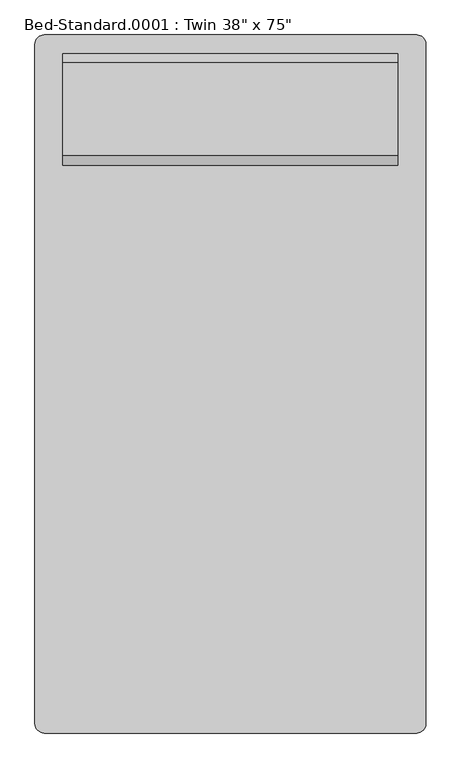
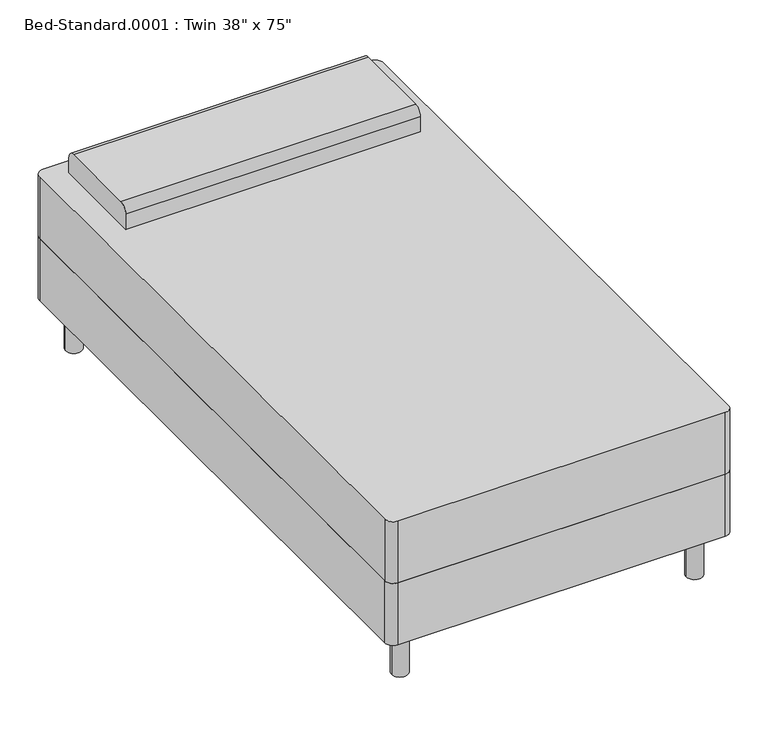
"""IFC4 building model written with IfcOpenShell, lengths in millimetres: furniture geometry."""

from ifc_helpers import new_model, si_unit, point, frame, frame_2d, origin, origin_with_axes, place, context, project, spatial, polyline, circle_curve, trimmed, segment, composite_curve, outline, extrude, source, transform, mapped, element, save


def furniture_c3d8c53b(model_context):
    return source(origin(), model_context, "Body", "SweptSolid", [
        extrude(outline(composite_curve([segment(polyline([(-261.9114754, -972.695082), (-261.9114754, 881.504918)]), True, "CONTINUOUS"), segment(trimmed(circle_curve(frame_2d((-236.5114754, 881.504918)), 25.4), [point((-261.9114754, 881.504918))], [point((-236.5114754, 906.904918))], False, "CARTESIAN"), True, "CONTINUOUS"), segment(polyline([(-236.5114754, 906.904918), (779.4885246, 906.904918)]), True, "CONTINUOUS"), segment(trimmed(circle_curve(frame_2d((779.4885246, 881.504918)), 25.4), [point((779.4885246, 906.904918))], [point((804.8885246, 881.504918))], False, "CARTESIAN"), True, "CONTINUOUS"), segment(polyline([(804.8885246, 881.504918), (804.8885246, -972.695082)]), True, "CONTINUOUS"), segment(trimmed(circle_curve(frame_2d((779.4885246, -972.695082)), 25.4), [point((804.8885246, -972.695082))], [point((779.4885246, -998.095082))], False, "CARTESIAN"), True, "CONTINUOUS"), segment(polyline([(779.4885246, -998.095082), (-236.5114754, -998.095082)]), True, "CONTINUOUS"), segment(trimmed(circle_curve(frame_2d((-236.5114754, -972.695082)), 25.4), [point((-236.5114754, -998.095082))], [point((-261.9114754, -972.695082))], False, "CARTESIAN"), True, "CONTINUOUS")], self_intersect=False)), frame((0.0, 0.0, 152.4), z_axis=(0.0, 0.0, 1.0), x_axis=(1.0, 0.0, 0.0)), (0.0, 0.0, 1.0), 203.2),
        extrude(outline(composite_curve([segment(polyline([(551.304918, 558.8), (551.304918, 609.6)]), True, "CONTINUOUS"), segment(trimmed(circle_curve(frame_2d((576.704918, 609.6)), 25.4), [point((551.304918, 609.6))], [point((576.704918, 635.0))], False, "CARTESIAN"), True, "CONTINUOUS"), segment(polyline([(576.704918, 635.0), (830.704918, 635.0)]), True, "CONTINUOUS"), segment(trimmed(circle_curve(frame_2d((830.704918, 609.6)), 25.4), [point((830.704918, 635.0))], [point((856.104918, 609.6))], False, "CARTESIAN"), True, "CONTINUOUS"), segment(polyline([(856.104918, 609.6), (856.104918, 558.8), (551.304918, 558.8)]), True, "CONTINUOUS")], self_intersect=False)), frame((-185.7114754, 0.0, 0.0), z_axis=(1.0, 0.0, 0.0), x_axis=(0.0, 1.0, 0.0)), (0.0, 0.0, 1.0), 914.4),
        extrude(outline(composite_curve([segment(trimmed(circle_curve(frame_2d((-185.7114754, 830.704918)), 25.4), [point((-211.1114754, 830.704918))], [point((-160.3114754, 830.704918))], False, "CARTESIAN"), True, "CONTINUOUS"), segment(trimmed(circle_curve(frame_2d((-185.7114754, 830.704918)), 25.4), [point((-160.3114754, 830.704918))], [point((-211.1114754, 830.704918))], False, "CARTESIAN"), True, "CONTINUOUS")], self_intersect=False)), origin_with_axes(), (0.0, 0.0, 1.0), 152.4),
        extrude(outline(composite_curve([segment(trimmed(circle_curve(frame_2d((728.6885246, 830.704918)), 25.4), [point((703.2885246, 830.704918))], [point((754.0885246, 830.704918))], False, "CARTESIAN"), True, "CONTINUOUS"), segment(trimmed(circle_curve(frame_2d((728.6885246, 830.704918)), 25.4), [point((754.0885246, 830.704918))], [point((703.2885246, 830.704918))], False, "CARTESIAN"), True, "CONTINUOUS")], self_intersect=False)), origin_with_axes(), (0.0, 0.0, 1.0), 152.4),
        extrude(outline(composite_curve([segment(trimmed(circle_curve(frame_2d((728.6885246, -921.895082)), 25.4), [point((703.2885246, -921.895082))], [point((754.0885246, -921.895082))], False, "CARTESIAN"), True, "CONTINUOUS"), segment(trimmed(circle_curve(frame_2d((728.6885246, -921.895082)), 25.4), [point((754.0885246, -921.895082))], [point((703.2885246, -921.895082))], False, "CARTESIAN"), True, "CONTINUOUS")], self_intersect=False)), origin_with_axes(), (0.0, 0.0, 1.0), 152.4),
        extrude(outline(composite_curve([segment(trimmed(circle_curve(frame_2d((-185.7114754, -921.895082)), 25.4), [point((-211.1114754, -921.895082))], [point((-160.3114754, -921.895082))], False, "CARTESIAN"), True, "CONTINUOUS"), segment(trimmed(circle_curve(frame_2d((-185.7114754, -921.895082)), 25.4), [point((-160.3114754, -921.895082))], [point((-211.1114754, -921.895082))], False, "CARTESIAN"), True, "CONTINUOUS")], self_intersect=False)), origin_with_axes(), (0.0, 0.0, 1.0), 152.4),
        extrude(outline(composite_curve([segment(polyline([(-236.5114754, 906.904918), (779.4885246, 906.904918)]), True, "CONTINUOUS"), segment(trimmed(circle_curve(frame_2d((779.4885246, 881.504918)), 25.4), [point((779.4885246, 906.904918))], [point((804.8885246, 881.504918))], False, "CARTESIAN"), True, "CONTINUOUS"), segment(polyline([(804.8885246, 881.504918), (804.8885246, -972.695082)]), True, "CONTINUOUS"), segment(trimmed(circle_curve(frame_2d((779.4885246, -972.695082)), 25.4), [point((804.8885246, -972.695082))], [point((779.4885246, -998.095082))], False, "CARTESIAN"), True, "CONTINUOUS"), segment(polyline([(779.4885246, -998.095082), (-236.5114754, -998.095082)]), True, "CONTINUOUS"), segment(trimmed(circle_curve(frame_2d((-236.5114754, -972.695082)), 25.4), [point((-236.5114754, -998.095082))], [point((-261.9114754, -972.695082))], False, "CARTESIAN"), True, "CONTINUOUS"), segment(polyline([(-261.9114754, -972.695082), (-261.9114754, 881.504918)]), True, "CONTINUOUS"), segment(trimmed(circle_curve(frame_2d((-236.5114754, 881.504918)), 25.4), [point((-261.9114754, 881.504918))], [point((-236.5114754, 906.904918))], False, "CARTESIAN"), True, "CONTINUOUS")], self_intersect=False)), frame((0.0, 0.0, 355.6), z_axis=(0.0, 0.0, 1.0), x_axis=(1.0, 0.0, 0.0)), (0.0, 0.0, 1.0), 203.2),
    ])


if __name__ == "__main__":
    model = new_model("IFC4")
    model_context = context("Model", 3, world=origin())
    ifc_project = project(units=[si_unit("LENGTHUNIT", "METRE", prefix="MILLI")], contexts=[model_context])
    site = spatial("IfcSite", under=ifc_project)
    building = spatial("IfcBuilding", under=site)
    placement = place(None, origin())
    furniture_shape = furniture_c3d8c53b(model_context)
    element("IfcFurniture", 1, ObjectType="Bed-Standard.0001 : Twin 38\" x 75\"", at=placement, inside=building, context=model_context, shape_type="MappedRepresentation", body=[
        mapped(furniture_shape, transform((0.0, 0.0, 0.0), x_axis=(1.0, 0.0, 0.0), y_axis=(0.0, 1.0, 0.0), z_axis=(0.0, 0.0, 1.0))),
    ])
    save(model, "model.ifc")

# Revit data of these elements
# Type "Bed-Standard.0001 : Twin 38\" x 75\""
#   Assembly Code = "E2020200"
#   Length = 6' - 3"
#   Width = 3' - 6"
#   Leg Material = Steel, Chrome Plated
#   Mattress Material = Linen, White
#   Default Elevation = 0
# Element 1 (IfcFurniture, "Bed-Standard.0001 : Twin 38\" x 75\"")
#   Materials on its faces: "Linen, White", "Steel, Chrome Plated"
# Materials
#   "Steel, Chrome Plated": class "Metal", colour RGB 17 17 17, transparency 0, Description = "Chromiuim plated steel", Cost = 0
#   "Linen, White": class "Textile", colour RGB 247 247 239, transparency 0, Description = "Linen, white", Cost = 0
